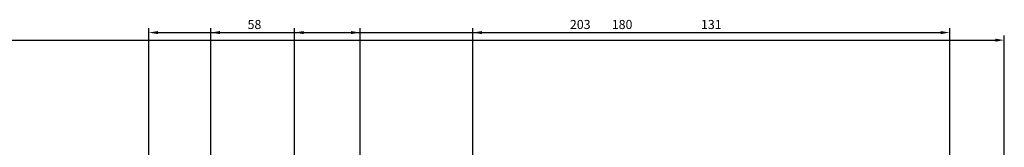
# Model space of a CAD drawing. Units: inches. Extents: x 604 to 3492, y -123 to 1737.
# Tile 19 of 20: x 1979 to 2250, y 1327 to 1362. Entities that reach past the tile are written whole.
import ezdxf

# ---------------------------------------------------------------- set-up
doc = ezdxf.new("R2010")
doc.units = ezdxf.units.IN
doc.layers.add('A-ANNO-DIMS', color=2, linetype='Continuous', lineweight=18)
doc.styles.get("Standard").update_dxf_attribs({"font": 'arial.ttf'})
doc.dimstyles.new('ISO-25', dxfattribs={"dimtxt": 2.5, "dimasz": 2.5, "dimexe": 1.25, "dimexo": 0.625, "dimtad": 1, "dimtxsty": 'Standard', "dimcen": 2.5, "dimadec": 0, "dimazin": 0, "dimtfac": 1, "dimtmove": 0, "dimatfit": 3, "dimfxl": 1, "dimarcsym": 0})

# ---------------------------------------------------------------- blocks, each defined once
blk = doc.blocks.new('*D71')
at = {"layer": 'A-ANNO-DIMS', "color": 0, "lineweight": -2, "transparency": 16777216}
for p, q in [((1574.57, 1288.33), (1574.57, 1357.82)), ((1577.07, 1356.57), (2247.07, 1356.57)), ((2249.57, 1288.33), (2249.57, 1357.82))]:
    blk.add_line(p, q, dxfattribs=at)
at = {"layer": 'A-ANNO-DIMS', "color": 0, "transparency": 16777216}
for points in [[(1577.07, 1356.98), (1577.07, 1356.15), (1574.57, 1356.57)], [(2247.07, 1356.98), (2247.07, 1356.15), (2249.57, 1356.57)]]:
    blk.add_solid(points, dxfattribs=at)
at = {"layer": 'Defpoints', "color": 0, "transparency": 16777216}
for p in [(2249.57, 1356.57), (1574.57, 1287.7), (2249.57, 1287.7)]:
    blk.add_point(p, dxfattribs=at)
at = {"layer": 'A-ANNO-DIMS', "color": 0, "transparency": 16777216, "insert": (1912.07, 1358.47), "char_height": 2.5, "attachment_point": 5}
blk.add_mtext('675', dxfattribs=at)
blk = doc.blocks.new('*D101')
at = {"layer": 'A-ANNO-DIMS', "color": 0, "lineweight": -2, "transparency": 16777216}
for p, q in [((2031.57, 843.33), (2031.57, 1359.9)), ((2034.07, 1358.65), (2232.07, 1358.65)), ((2234.57, 843.33), (2234.57, 1359.9))]:
    blk.add_line(p, q, dxfattribs=at)
at = {"layer": 'A-ANNO-DIMS', "color": 0, "transparency": 16777216}
for points in [[(2034.07, 1359.07), (2034.07, 1358.23), (2031.57, 1358.65)], [(2232.07, 1359.07), (2232.07, 1358.23), (2234.57, 1358.65)]]:
    blk.add_solid(points, dxfattribs=at)
at = {"layer": 'Defpoints', "color": 0, "transparency": 16777216}
for p in [(2234.57, 1358.65), (2031.57, 842.7), (2234.57, 842.7)]:
    blk.add_point(p, dxfattribs=at)
at = {"layer": 'A-ANNO-DIMS', "color": 0, "transparency": 16777216, "insert": (2133.07, 1360.55), "char_height": 2.5, "attachment_point": 5}
blk.add_mtext('203', dxfattribs=at)
blk = doc.blocks.new('*D109')
at = {"layer": 'A-ANNO-DIMS', "color": 0, "lineweight": -2, "transparency": 16777216}
for p, q in [((2054.57, 740.33), (2054.57, 1359.9)), ((2057.07, 1358.65), (2232.07, 1358.65)), ((2234.57, 740.33), (2234.57, 1359.9))]:
    blk.add_line(p, q, dxfattribs=at)
at = {"layer": 'A-ANNO-DIMS', "color": 0, "transparency": 16777216}
for points in [[(2057.07, 1359.07), (2057.07, 1358.23), (2054.57, 1358.65)], [(2232.07, 1359.07), (2232.07, 1358.23), (2234.57, 1358.65)]]:
    blk.add_solid(points, dxfattribs=at)
at = {"layer": 'Defpoints', "color": 0, "transparency": 16777216}
for p in [(2234.57, 1358.65), (2054.57, 739.7), (2234.57, 739.7)]:
    blk.add_point(p, dxfattribs=at)
at = {"layer": 'A-ANNO-DIMS', "color": 0, "transparency": 16777216, "insert": (2144.57, 1360.55), "char_height": 2.5, "attachment_point": 5}
blk.add_mtext('180', dxfattribs=at)
blk = doc.blocks.new('*D111')
at = {"layer": 'A-ANNO-DIMS', "color": 0, "lineweight": -2, "transparency": 16777216}
for p, q in [((2103.57, 973.33), (2103.57, 1359.9)), ((2106.07, 1358.65), (2232.07, 1358.65)), ((2234.57, 973.33), (2234.57, 1359.9))]:
    blk.add_line(p, q, dxfattribs=at)
at = {"layer": 'A-ANNO-DIMS', "color": 0, "transparency": 16777216}
for points in [[(2106.07, 1359.07), (2106.07, 1358.23), (2103.57, 1358.65)], [(2232.07, 1359.07), (2232.07, 1358.23), (2234.57, 1358.65)]]:
    blk.add_solid(points, dxfattribs=at)
at = {"layer": 'Defpoints', "color": 0, "transparency": 16777216}
for p in [(2234.57, 1358.65), (2103.57, 972.7), (2234.57, 972.7)]:
    blk.add_point(p, dxfattribs=at)
at = {"layer": 'A-ANNO-DIMS', "color": 0, "transparency": 16777216, "insert": (2169.07, 1360.55), "char_height": 2.5, "attachment_point": 5}
blk.add_mtext('131', dxfattribs=at)
blk = doc.blocks.new('*D113')
at = {"layer": 'A-ANNO-DIMS', "color": 0, "lineweight": -2, "transparency": 16777216}
for p, q in [((2014.57, 603.33), (2014.57, 1359.9)), ((2017.07, 1358.65), (2070.07, 1358.65)), ((2072.57, 603.33), (2072.57, 1359.9))]:
    blk.add_line(p, q, dxfattribs=at)
at = {"layer": 'A-ANNO-DIMS', "color": 0, "transparency": 16777216}
for points in [[(2017.07, 1359.07), (2017.07, 1358.23), (2014.57, 1358.65)], [(2070.07, 1359.07), (2070.07, 1358.23), (2072.57, 1358.65)]]:
    blk.add_solid(points, dxfattribs=at)
at = {"layer": 'Defpoints', "color": 0, "transparency": 16777216}
for p in [(2072.57, 1358.65), (2014.57, 602.7), (2072.57, 602.7)]:
    blk.add_point(p, dxfattribs=at)
at = {"layer": 'A-ANNO-DIMS', "color": 0, "transparency": 16777216, "insert": (2043.57, 1360.55), "char_height": 2.5, "attachment_point": 5}
blk.add_mtext('58', dxfattribs=at)

msp = doc.modelspace()

# ---------------------------------------------------------------- dimensions: what is measured, and where the dimension line sits
at = {"layer": 'A-ANNO-DIMS'}
for base, p1, p2, picture, middle in [((2072.5743, 1358.6504), (2014.5743, 602.7004), (2072.5743, 602.7004), '*D113', (2043.5743, 1360.5519)), ((2234.5743, 1358.6504), (2031.5743, 842.7004), (2234.5743, 842.7004), '*D101', (2133.0743, 1360.5527)), ((2234.5743, 1358.6504), (2054.5743, 739.7004), (2234.5743, 739.7004), '*D109', (2144.5743, 1360.5519)), ((2234.5743, 1358.6504), (2103.5743, 972.7004), (2234.5743, 972.7004), '*D111', (2169.0743, 1360.5527))]:
    dim = msp.add_linear_dim(base=base, p1=p1, p2=p2, dimstyle='ISO-25', override={"dimdec": 0, "dimlfac": 1, "dimrnd": 0, "dimzin": 0, "dimdsep": 46, "dimlunit": 2}, dxfattribs=at)
    dim.commit()
    dim.dimension.update_dxf_attribs({"geometry": picture, "text_midpoint": middle})
dim = msp.add_aligned_dim(p1=(1574.5743, 1287.7004), p2=(2249.5743, 1287.7004), distance=68.8648, dimstyle='ISO-25', override={"dimclrd": 0, "dimclre": 0, "dimclrt": 0}, dxfattribs=at)
dim.commit()
dim.dimension.update_dxf_attribs({"geometry": '*D71', "text_midpoint": (1912.0743, 1358.4667)})

doc.saveas('drawing.dxf')
